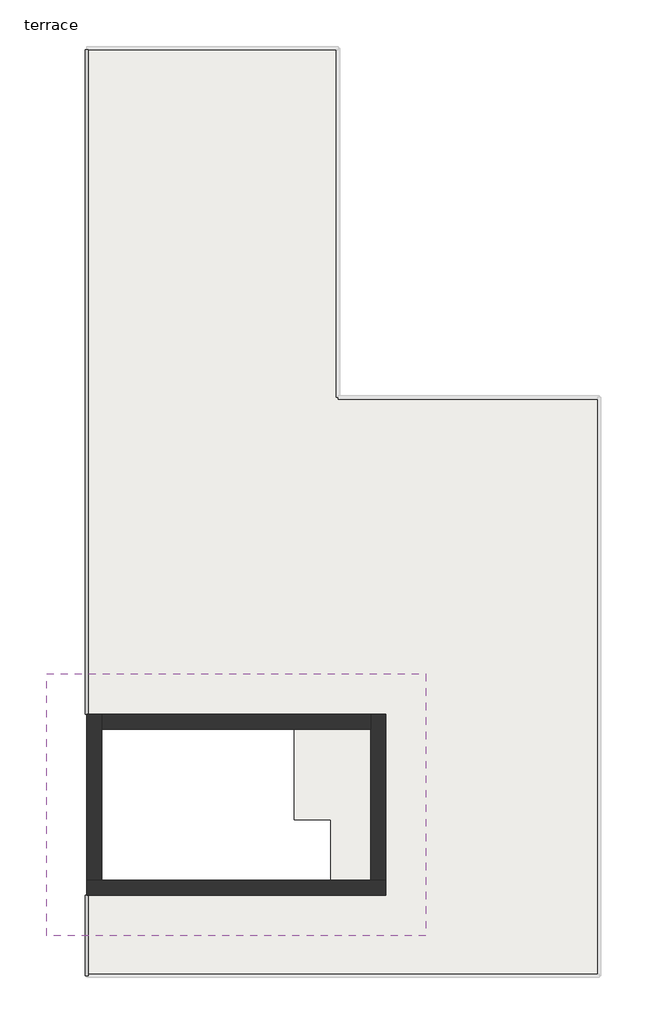
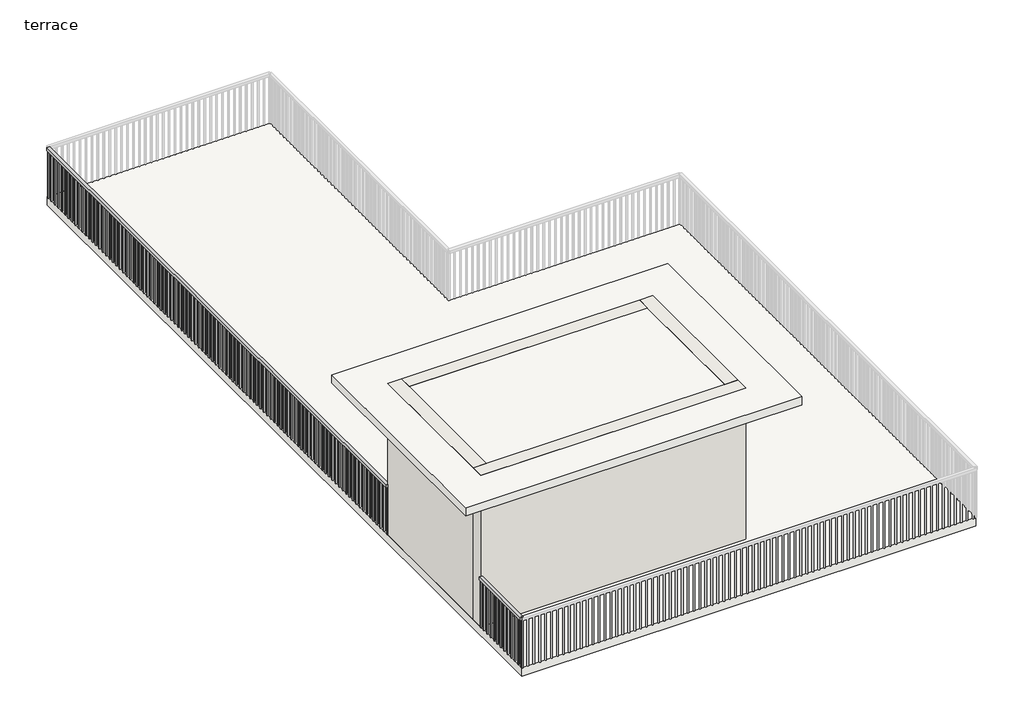
# One storey, part 1 of 4: 4 walls, 2 railings, 2 slabs.
"""IFC4 building model written with IfcOpenShell, lengths in millimetres."""

from ifc_helpers import new_model, si_unit, frame, origin, place, context, project, spatial, polyline, outline, extrude, faceted_brep, element, save

model = new_model("IFC4")

# Units and contexts
model_context = context("Model", 3, world=origin())
ifc_project = project(units=[si_unit("LENGTHUNIT", "METRE", prefix="MILLI")], contexts=[model_context])

# Site, building, storey
site = spatial("IfcSite", under=ifc_project)
building = spatial("IfcBuilding", under=site)
storey = spatial("IfcBuildingStorey", under=building, Name="terrace", Elevation=7010.4)

# Railings
placement = place(None, origin())
element("IfcRailing", 1, ObjectType="Handrail - Rectangular", at=placement, inside=storey, context=model_context, shape_type="SweptSolid", body=[
    extrude(outline(polyline([(28356.9316163, 19632.8980552), (28407.7316163, 19632.8980552), (28407.7316163, 9561.7980552), (28356.9316163, 9561.7980552), (28356.9316163, 19632.8980552)])), frame((0.0, 0.0, 7874.0), z_axis=(0.0, 0.0, 1.0), x_axis=(1.0, 0.0, 0.0)), (0.0, 0.0, 1.0), 50.8),
    extrude(outline(polyline([(28372.8066163, 9584.0230552), (28391.8566163, 9584.0230552), (28391.8566163, 9564.9730552), (28372.8066163, 9564.9730552), (28372.8066163, 9584.0230552)])), frame((0.0, 0.0, 7010.4), z_axis=(0.0, 0.0, 1.0), x_axis=(1.0, 0.0, 0.0)), (0.0, 0.0, 1.0), 863.6),
    extrude(outline(polyline([(28372.8066163, 9685.6230552), (28391.8566163, 9685.6230552), (28391.8566163, 9666.5730552), (28372.8066163, 9666.5730552), (28372.8066163, 9685.6230552)])), frame((0.0, 0.0, 7010.4), z_axis=(0.0, 0.0, 1.0), x_axis=(1.0, 0.0, 0.0)), (0.0, 0.0, 1.0), 863.6),
    extrude(outline(polyline([(28372.8066163, 9787.2230552), (28391.8566163, 9787.2230552), (28391.8566163, 9768.1730552), (28372.8066163, 9768.1730552), (28372.8066163, 9787.2230552)])), frame((0.0, 0.0, 7010.4), z_axis=(0.0, 0.0, 1.0), x_axis=(1.0, 0.0, 0.0)), (0.0, 0.0, 1.0), 863.6),
    extrude(outline(polyline([(28372.8066163, 9888.8230552), (28391.8566163, 9888.8230552), (28391.8566163, 9869.7730552), (28372.8066163, 9869.7730552), (28372.8066163, 9888.8230552)])), frame((0.0, 0.0, 7010.4), z_axis=(0.0, 0.0, 1.0), x_axis=(1.0, 0.0, 0.0)), (0.0, 0.0, 1.0), 863.6),
    extrude(outline(polyline([(28372.8066163, 9990.4230552), (28391.8566163, 9990.4230552), (28391.8566163, 9971.3730552), (28372.8066163, 9971.3730552), (28372.8066163, 9990.4230552)])), frame((0.0, 0.0, 7010.4), z_axis=(0.0, 0.0, 1.0), x_axis=(1.0, 0.0, 0.0)), (0.0, 0.0, 1.0), 863.6),
    extrude(outline(polyline([(28372.8066163, 10092.0230552), (28391.8566163, 10092.0230552), (28391.8566163, 10072.9730552), (28372.8066163, 10072.9730552), (28372.8066163, 10092.0230552)])), frame((0.0, 0.0, 7010.4), z_axis=(0.0, 0.0, 1.0), x_axis=(1.0, 0.0, 0.0)), (0.0, 0.0, 1.0), 863.6),
    extrude(outline(polyline([(28372.8066163, 10193.6230552), (28391.8566163, 10193.6230552), (28391.8566163, 10174.5730552), (28372.8066163, 10174.5730552), (28372.8066163, 10193.6230552)])), frame((0.0, 0.0, 7010.4), z_axis=(0.0, 0.0, 1.0), x_axis=(1.0, 0.0, 0.0)), (0.0, 0.0, 1.0), 863.6),
    extrude(outline(polyline([(28372.8066163, 10295.2230552), (28391.8566163, 10295.2230552), (28391.8566163, 10276.1730552), (28372.8066163, 10276.1730552), (28372.8066163, 10295.2230552)])), frame((0.0, 0.0, 7010.4), z_axis=(0.0, 0.0, 1.0), x_axis=(1.0, 0.0, 0.0)), (0.0, 0.0, 1.0), 863.6),
    extrude(outline(polyline([(28372.8066163, 10396.8230552), (28391.8566163, 10396.8230552), (28391.8566163, 10377.7730552), (28372.8066163, 10377.7730552), (28372.8066163, 10396.8230552)])), frame((0.0, 0.0, 7010.4), z_axis=(0.0, 0.0, 1.0), x_axis=(1.0, 0.0, 0.0)), (0.0, 0.0, 1.0), 863.6),
    extrude(outline(polyline([(28372.8066163, 10498.4230552), (28391.8566163, 10498.4230552), (28391.8566163, 10479.3730552), (28372.8066163, 10479.3730552), (28372.8066163, 10498.4230552)])), frame((0.0, 0.0, 7010.4), z_axis=(0.0, 0.0, 1.0), x_axis=(1.0, 0.0, 0.0)), (0.0, 0.0, 1.0), 863.6),
    extrude(outline(polyline([(28372.8066163, 10600.0230552), (28391.8566163, 10600.0230552), (28391.8566163, 10580.9730552), (28372.8066163, 10580.9730552), (28372.8066163, 10600.0230552)])), frame((0.0, 0.0, 7010.4), z_axis=(0.0, 0.0, 1.0), x_axis=(1.0, 0.0, 0.0)), (0.0, 0.0, 1.0), 863.6),
    extrude(outline(polyline([(28372.8066163, 10701.6230552), (28391.8566163, 10701.6230552), (28391.8566163, 10682.5730552), (28372.8066163, 10682.5730552), (28372.8066163, 10701.6230552)])), frame((0.0, 0.0, 7010.4), z_axis=(0.0, 0.0, 1.0), x_axis=(1.0, 0.0, 0.0)), (0.0, 0.0, 1.0), 863.6),
    extrude(outline(polyline([(28372.8066163, 10803.2230552), (28391.8566163, 10803.2230552), (28391.8566163, 10784.1730552), (28372.8066163, 10784.1730552), (28372.8066163, 10803.2230552)])), frame((0.0, 0.0, 7010.4), z_axis=(0.0, 0.0, 1.0), x_axis=(1.0, 0.0, 0.0)), (0.0, 0.0, 1.0), 863.6),
    extrude(outline(polyline([(28372.8066163, 10904.8230552), (28391.8566163, 10904.8230552), (28391.8566163, 10885.7730552), (28372.8066163, 10885.7730552), (28372.8066163, 10904.8230552)])), frame((0.0, 0.0, 7010.4), z_axis=(0.0, 0.0, 1.0), x_axis=(1.0, 0.0, 0.0)), (0.0, 0.0, 1.0), 863.6),
    extrude(outline(polyline([(28372.8066163, 11006.4230552), (28391.8566163, 11006.4230552), (28391.8566163, 10987.3730552), (28372.8066163, 10987.3730552), (28372.8066163, 11006.4230552)])), frame((0.0, 0.0, 7010.4), z_axis=(0.0, 0.0, 1.0), x_axis=(1.0, 0.0, 0.0)), (0.0, 0.0, 1.0), 863.6),
    extrude(outline(polyline([(28372.8066163, 11108.0230552), (28391.8566163, 11108.0230552), (28391.8566163, 11088.9730552), (28372.8066163, 11088.9730552), (28372.8066163, 11108.0230552)])), frame((0.0, 0.0, 7010.4), z_axis=(0.0, 0.0, 1.0), x_axis=(1.0, 0.0, 0.0)), (0.0, 0.0, 1.0), 863.6),
    extrude(outline(polyline([(28372.8066163, 11209.6230552), (28391.8566163, 11209.6230552), (28391.8566163, 11190.5730552), (28372.8066163, 11190.5730552), (28372.8066163, 11209.6230552)])), frame((0.0, 0.0, 7010.4), z_axis=(0.0, 0.0, 1.0), x_axis=(1.0, 0.0, 0.0)), (0.0, 0.0, 1.0), 863.6),
    extrude(outline(polyline([(28372.8066163, 11311.2230552), (28391.8566163, 11311.2230552), (28391.8566163, 11292.1730552), (28372.8066163, 11292.1730552), (28372.8066163, 11311.2230552)])), frame((0.0, 0.0, 7010.4), z_axis=(0.0, 0.0, 1.0), x_axis=(1.0, 0.0, 0.0)), (0.0, 0.0, 1.0), 863.6),
    extrude(outline(polyline([(28372.8066163, 11412.8230552), (28391.8566163, 11412.8230552), (28391.8566163, 11393.7730552), (28372.8066163, 11393.7730552), (28372.8066163, 11412.8230552)])), frame((0.0, 0.0, 7010.4), z_axis=(0.0, 0.0, 1.0), x_axis=(1.0, 0.0, 0.0)), (0.0, 0.0, 1.0), 863.6),
    extrude(outline(polyline([(28372.8066163, 11514.4230552), (28391.8566163, 11514.4230552), (28391.8566163, 11495.3730552), (28372.8066163, 11495.3730552), (28372.8066163, 11514.4230552)])), frame((0.0, 0.0, 7010.4), z_axis=(0.0, 0.0, 1.0), x_axis=(1.0, 0.0, 0.0)), (0.0, 0.0, 1.0), 863.6),
    extrude(outline(polyline([(28372.8066163, 11616.0230552), (28391.8566163, 11616.0230552), (28391.8566163, 11596.9730552), (28372.8066163, 11596.9730552), (28372.8066163, 11616.0230552)])), frame((0.0, 0.0, 7010.4), z_axis=(0.0, 0.0, 1.0), x_axis=(1.0, 0.0, 0.0)), (0.0, 0.0, 1.0), 863.6),
    extrude(outline(polyline([(28372.8066163, 11717.6230552), (28391.8566163, 11717.6230552), (28391.8566163, 11698.5730552), (28372.8066163, 11698.5730552), (28372.8066163, 11717.6230552)])), frame((0.0, 0.0, 7010.4), z_axis=(0.0, 0.0, 1.0), x_axis=(1.0, 0.0, 0.0)), (0.0, 0.0, 1.0), 863.6),
    extrude(outline(polyline([(28372.8066163, 11819.2230552), (28391.8566163, 11819.2230552), (28391.8566163, 11800.1730552), (28372.8066163, 11800.1730552), (28372.8066163, 11819.2230552)])), frame((0.0, 0.0, 7010.4), z_axis=(0.0, 0.0, 1.0), x_axis=(1.0, 0.0, 0.0)), (0.0, 0.0, 1.0), 863.6),
    extrude(outline(polyline([(28372.8066163, 11920.8230552), (28391.8566163, 11920.8230552), (28391.8566163, 11901.7730552), (28372.8066163, 11901.7730552), (28372.8066163, 11920.8230552)])), frame((0.0, 0.0, 7010.4), z_axis=(0.0, 0.0, 1.0), x_axis=(1.0, 0.0, 0.0)), (0.0, 0.0, 1.0), 863.6),
    extrude(outline(polyline([(28372.8066163, 12022.4230552), (28391.8566163, 12022.4230552), (28391.8566163, 12003.3730552), (28372.8066163, 12003.3730552), (28372.8066163, 12022.4230552)])), frame((0.0, 0.0, 7010.4), z_axis=(0.0, 0.0, 1.0), x_axis=(1.0, 0.0, 0.0)), (0.0, 0.0, 1.0), 863.6),
    extrude(outline(polyline([(28372.8066163, 12124.0230552), (28391.8566163, 12124.0230552), (28391.8566163, 12104.9730552), (28372.8066163, 12104.9730552), (28372.8066163, 12124.0230552)])), frame((0.0, 0.0, 7010.4), z_axis=(0.0, 0.0, 1.0), x_axis=(1.0, 0.0, 0.0)), (0.0, 0.0, 1.0), 863.6),
    extrude(outline(polyline([(28372.8066163, 12225.6230552), (28391.8566163, 12225.6230552), (28391.8566163, 12206.5730552), (28372.8066163, 12206.5730552), (28372.8066163, 12225.6230552)])), frame((0.0, 0.0, 7010.4), z_axis=(0.0, 0.0, 1.0), x_axis=(1.0, 0.0, 0.0)), (0.0, 0.0, 1.0), 863.6),
    extrude(outline(polyline([(28372.8066163, 12327.2230552), (28391.8566163, 12327.2230552), (28391.8566163, 12308.1730552), (28372.8066163, 12308.1730552), (28372.8066163, 12327.2230552)])), frame((0.0, 0.0, 7010.4), z_axis=(0.0, 0.0, 1.0), x_axis=(1.0, 0.0, 0.0)), (0.0, 0.0, 1.0), 863.6),
    extrude(outline(polyline([(28372.8066163, 12428.8230552), (28391.8566163, 12428.8230552), (28391.8566163, 12409.7730552), (28372.8066163, 12409.7730552), (28372.8066163, 12428.8230552)])), frame((0.0, 0.0, 7010.4), z_axis=(0.0, 0.0, 1.0), x_axis=(1.0, 0.0, 0.0)), (0.0, 0.0, 1.0), 863.6),
    extrude(outline(polyline([(28372.8066163, 12530.4230552), (28391.8566163, 12530.4230552), (28391.8566163, 12511.3730552), (28372.8066163, 12511.3730552), (28372.8066163, 12530.4230552)])), frame((0.0, 0.0, 7010.4), z_axis=(0.0, 0.0, 1.0), x_axis=(1.0, 0.0, 0.0)), (0.0, 0.0, 1.0), 863.6),
    extrude(outline(polyline([(28372.8066163, 12632.0230552), (28391.8566163, 12632.0230552), (28391.8566163, 12612.9730552), (28372.8066163, 12612.9730552), (28372.8066163, 12632.0230552)])), frame((0.0, 0.0, 7010.4), z_axis=(0.0, 0.0, 1.0), x_axis=(1.0, 0.0, 0.0)), (0.0, 0.0, 1.0), 863.6),
    extrude(outline(polyline([(28372.8066163, 12733.6230552), (28391.8566163, 12733.6230552), (28391.8566163, 12714.5730552), (28372.8066163, 12714.5730552), (28372.8066163, 12733.6230552)])), frame((0.0, 0.0, 7010.4), z_axis=(0.0, 0.0, 1.0), x_axis=(1.0, 0.0, 0.0)), (0.0, 0.0, 1.0), 863.6),
    extrude(outline(polyline([(28372.8066163, 12835.2230552), (28391.8566163, 12835.2230552), (28391.8566163, 12816.1730552), (28372.8066163, 12816.1730552), (28372.8066163, 12835.2230552)])), frame((0.0, 0.0, 7010.4), z_axis=(0.0, 0.0, 1.0), x_axis=(1.0, 0.0, 0.0)), (0.0, 0.0, 1.0), 863.6),
    extrude(outline(polyline([(28372.8066163, 12936.8230552), (28391.8566163, 12936.8230552), (28391.8566163, 12917.7730552), (28372.8066163, 12917.7730552), (28372.8066163, 12936.8230552)])), frame((0.0, 0.0, 7010.4), z_axis=(0.0, 0.0, 1.0), x_axis=(1.0, 0.0, 0.0)), (0.0, 0.0, 1.0), 863.6),
    extrude(outline(polyline([(28372.8066163, 13038.4230552), (28391.8566163, 13038.4230552), (28391.8566163, 13019.3730552), (28372.8066163, 13019.3730552), (28372.8066163, 13038.4230552)])), frame((0.0, 0.0, 7010.4), z_axis=(0.0, 0.0, 1.0), x_axis=(1.0, 0.0, 0.0)), (0.0, 0.0, 1.0), 863.6),
    extrude(outline(polyline([(28372.8066163, 13140.0230552), (28391.8566163, 13140.0230552), (28391.8566163, 13120.9730552), (28372.8066163, 13120.9730552), (28372.8066163, 13140.0230552)])), frame((0.0, 0.0, 7010.4), z_axis=(0.0, 0.0, 1.0), x_axis=(1.0, 0.0, 0.0)), (0.0, 0.0, 1.0), 863.6),
    extrude(outline(polyline([(28372.8066163, 13241.6230552), (28391.8566163, 13241.6230552), (28391.8566163, 13222.5730552), (28372.8066163, 13222.5730552), (28372.8066163, 13241.6230552)])), frame((0.0, 0.0, 7010.4), z_axis=(0.0, 0.0, 1.0), x_axis=(1.0, 0.0, 0.0)), (0.0, 0.0, 1.0), 863.6),
    extrude(outline(polyline([(28372.8066163, 13343.2230552), (28391.8566163, 13343.2230552), (28391.8566163, 13324.1730552), (28372.8066163, 13324.1730552), (28372.8066163, 13343.2230552)])), frame((0.0, 0.0, 7010.4), z_axis=(0.0, 0.0, 1.0), x_axis=(1.0, 0.0, 0.0)), (0.0, 0.0, 1.0), 863.6),
    extrude(outline(polyline([(28372.8066163, 13444.8230552), (28391.8566163, 13444.8230552), (28391.8566163, 13425.7730552), (28372.8066163, 13425.7730552), (28372.8066163, 13444.8230552)])), frame((0.0, 0.0, 7010.4), z_axis=(0.0, 0.0, 1.0), x_axis=(1.0, 0.0, 0.0)), (0.0, 0.0, 1.0), 863.6),
    extrude(outline(polyline([(28372.8066163, 13546.4230552), (28391.8566163, 13546.4230552), (28391.8566163, 13527.3730552), (28372.8066163, 13527.3730552), (28372.8066163, 13546.4230552)])), frame((0.0, 0.0, 7010.4), z_axis=(0.0, 0.0, 1.0), x_axis=(1.0, 0.0, 0.0)), (0.0, 0.0, 1.0), 863.6),
    extrude(outline(polyline([(28372.8066163, 13648.0230552), (28391.8566163, 13648.0230552), (28391.8566163, 13628.9730552), (28372.8066163, 13628.9730552), (28372.8066163, 13648.0230552)])), frame((0.0, 0.0, 7010.4), z_axis=(0.0, 0.0, 1.0), x_axis=(1.0, 0.0, 0.0)), (0.0, 0.0, 1.0), 863.6),
    extrude(outline(polyline([(28372.8066163, 13749.6230552), (28391.8566163, 13749.6230552), (28391.8566163, 13730.5730552), (28372.8066163, 13730.5730552), (28372.8066163, 13749.6230552)])), frame((0.0, 0.0, 7010.4), z_axis=(0.0, 0.0, 1.0), x_axis=(1.0, 0.0, 0.0)), (0.0, 0.0, 1.0), 863.6),
    extrude(outline(polyline([(28372.8066163, 13851.2230552), (28391.8566163, 13851.2230552), (28391.8566163, 13832.1730552), (28372.8066163, 13832.1730552), (28372.8066163, 13851.2230552)])), frame((0.0, 0.0, 7010.4), z_axis=(0.0, 0.0, 1.0), x_axis=(1.0, 0.0, 0.0)), (0.0, 0.0, 1.0), 863.6),
    extrude(outline(polyline([(28372.8066163, 13952.8230552), (28391.8566163, 13952.8230552), (28391.8566163, 13933.7730552), (28372.8066163, 13933.7730552), (28372.8066163, 13952.8230552)])), frame((0.0, 0.0, 7010.4), z_axis=(0.0, 0.0, 1.0), x_axis=(1.0, 0.0, 0.0)), (0.0, 0.0, 1.0), 863.6),
    extrude(outline(polyline([(28372.8066163, 14054.4230552), (28391.8566163, 14054.4230552), (28391.8566163, 14035.3730552), (28372.8066163, 14035.3730552), (28372.8066163, 14054.4230552)])), frame((0.0, 0.0, 7010.4), z_axis=(0.0, 0.0, 1.0), x_axis=(1.0, 0.0, 0.0)), (0.0, 0.0, 1.0), 863.6),
    extrude(outline(polyline([(28372.8066163, 14156.0230552), (28391.8566163, 14156.0230552), (28391.8566163, 14136.9730552), (28372.8066163, 14136.9730552), (28372.8066163, 14156.0230552)])), frame((0.0, 0.0, 7010.4), z_axis=(0.0, 0.0, 1.0), x_axis=(1.0, 0.0, 0.0)), (0.0, 0.0, 1.0), 863.6),
    extrude(outline(polyline([(28372.8066163, 14257.6230552), (28391.8566163, 14257.6230552), (28391.8566163, 14238.5730552), (28372.8066163, 14238.5730552), (28372.8066163, 14257.6230552)])), frame((0.0, 0.0, 7010.4), z_axis=(0.0, 0.0, 1.0), x_axis=(1.0, 0.0, 0.0)), (0.0, 0.0, 1.0), 863.6),
    extrude(outline(polyline([(28372.8066163, 14359.2230552), (28391.8566163, 14359.2230552), (28391.8566163, 14340.1730552), (28372.8066163, 14340.1730552), (28372.8066163, 14359.2230552)])), frame((0.0, 0.0, 7010.4), z_axis=(0.0, 0.0, 1.0), x_axis=(1.0, 0.0, 0.0)), (0.0, 0.0, 1.0), 863.6),
    extrude(outline(polyline([(28372.8066163, 14460.8230552), (28391.8566163, 14460.8230552), (28391.8566163, 14441.7730552), (28372.8066163, 14441.7730552), (28372.8066163, 14460.8230552)])), frame((0.0, 0.0, 7010.4), z_axis=(0.0, 0.0, 1.0), x_axis=(1.0, 0.0, 0.0)), (0.0, 0.0, 1.0), 863.6),
    extrude(outline(polyline([(28372.8066163, 14562.4230552), (28391.8566163, 14562.4230552), (28391.8566163, 14543.3730552), (28372.8066163, 14543.3730552), (28372.8066163, 14562.4230552)])), frame((0.0, 0.0, 7010.4), z_axis=(0.0, 0.0, 1.0), x_axis=(1.0, 0.0, 0.0)), (0.0, 0.0, 1.0), 863.6),
    extrude(outline(polyline([(28372.8066163, 14664.0230552), (28391.8566163, 14664.0230552), (28391.8566163, 14644.9730552), (28372.8066163, 14644.9730552), (28372.8066163, 14664.0230552)])), frame((0.0, 0.0, 7010.4), z_axis=(0.0, 0.0, 1.0), x_axis=(1.0, 0.0, 0.0)), (0.0, 0.0, 1.0), 863.6),
    extrude(outline(polyline([(28372.8066163, 14765.6230552), (28391.8566163, 14765.6230552), (28391.8566163, 14746.5730552), (28372.8066163, 14746.5730552), (28372.8066163, 14765.6230552)])), frame((0.0, 0.0, 7010.4), z_axis=(0.0, 0.0, 1.0), x_axis=(1.0, 0.0, 0.0)), (0.0, 0.0, 1.0), 863.6),
    extrude(outline(polyline([(28372.8066163, 14867.2230552), (28391.8566163, 14867.2230552), (28391.8566163, 14848.1730552), (28372.8066163, 14848.1730552), (28372.8066163, 14867.2230552)])), frame((0.0, 0.0, 7010.4), z_axis=(0.0, 0.0, 1.0), x_axis=(1.0, 0.0, 0.0)), (0.0, 0.0, 1.0), 863.6),
    extrude(outline(polyline([(28372.8066163, 14968.8230552), (28391.8566163, 14968.8230552), (28391.8566163, 14949.7730552), (28372.8066163, 14949.7730552), (28372.8066163, 14968.8230552)])), frame((0.0, 0.0, 7010.4), z_axis=(0.0, 0.0, 1.0), x_axis=(1.0, 0.0, 0.0)), (0.0, 0.0, 1.0), 863.6),
    extrude(outline(polyline([(28372.8066163, 15070.4230552), (28391.8566163, 15070.4230552), (28391.8566163, 15051.3730552), (28372.8066163, 15051.3730552), (28372.8066163, 15070.4230552)])), frame((0.0, 0.0, 7010.4), z_axis=(0.0, 0.0, 1.0), x_axis=(1.0, 0.0, 0.0)), (0.0, 0.0, 1.0), 863.6),
    extrude(outline(polyline([(28372.8066163, 15172.0230552), (28391.8566163, 15172.0230552), (28391.8566163, 15152.9730552), (28372.8066163, 15152.9730552), (28372.8066163, 15172.0230552)])), frame((0.0, 0.0, 7010.4), z_axis=(0.0, 0.0, 1.0), x_axis=(1.0, 0.0, 0.0)), (0.0, 0.0, 1.0), 863.6),
    extrude(outline(polyline([(28372.8066163, 15273.6230552), (28391.8566163, 15273.6230552), (28391.8566163, 15254.5730552), (28372.8066163, 15254.5730552), (28372.8066163, 15273.6230552)])), frame((0.0, 0.0, 7010.4), z_axis=(0.0, 0.0, 1.0), x_axis=(1.0, 0.0, 0.0)), (0.0, 0.0, 1.0), 863.6),
    extrude(outline(polyline([(28372.8066163, 15375.2230552), (28391.8566163, 15375.2230552), (28391.8566163, 15356.1730552), (28372.8066163, 15356.1730552), (28372.8066163, 15375.2230552)])), frame((0.0, 0.0, 7010.4), z_axis=(0.0, 0.0, 1.0), x_axis=(1.0, 0.0, 0.0)), (0.0, 0.0, 1.0), 863.6),
    extrude(outline(polyline([(28372.8066163, 15476.8230552), (28391.8566163, 15476.8230552), (28391.8566163, 15457.7730552), (28372.8066163, 15457.7730552), (28372.8066163, 15476.8230552)])), frame((0.0, 0.0, 7010.4), z_axis=(0.0, 0.0, 1.0), x_axis=(1.0, 0.0, 0.0)), (0.0, 0.0, 1.0), 863.6),
    extrude(outline(polyline([(28372.8066163, 15578.4230552), (28391.8566163, 15578.4230552), (28391.8566163, 15559.3730552), (28372.8066163, 15559.3730552), (28372.8066163, 15578.4230552)])), frame((0.0, 0.0, 7010.4), z_axis=(0.0, 0.0, 1.0), x_axis=(1.0, 0.0, 0.0)), (0.0, 0.0, 1.0), 863.6),
    extrude(outline(polyline([(28372.8066163, 15680.0230552), (28391.8566163, 15680.0230552), (28391.8566163, 15660.9730552), (28372.8066163, 15660.9730552), (28372.8066163, 15680.0230552)])), frame((0.0, 0.0, 7010.4), z_axis=(0.0, 0.0, 1.0), x_axis=(1.0, 0.0, 0.0)), (0.0, 0.0, 1.0), 863.6),
    extrude(outline(polyline([(28372.8066163, 15781.6230552), (28391.8566163, 15781.6230552), (28391.8566163, 15762.5730552), (28372.8066163, 15762.5730552), (28372.8066163, 15781.6230552)])), frame((0.0, 0.0, 7010.4), z_axis=(0.0, 0.0, 1.0), x_axis=(1.0, 0.0, 0.0)), (0.0, 0.0, 1.0), 863.6),
    extrude(outline(polyline([(28372.8066163, 15883.2230552), (28391.8566163, 15883.2230552), (28391.8566163, 15864.1730552), (28372.8066163, 15864.1730552), (28372.8066163, 15883.2230552)])), frame((0.0, 0.0, 7010.4), z_axis=(0.0, 0.0, 1.0), x_axis=(1.0, 0.0, 0.0)), (0.0, 0.0, 1.0), 863.6),
    extrude(outline(polyline([(28372.8066163, 15984.8230552), (28391.8566163, 15984.8230552), (28391.8566163, 15965.7730552), (28372.8066163, 15965.7730552), (28372.8066163, 15984.8230552)])), frame((0.0, 0.0, 7010.4), z_axis=(0.0, 0.0, 1.0), x_axis=(1.0, 0.0, 0.0)), (0.0, 0.0, 1.0), 863.6),
    extrude(outline(polyline([(28372.8066163, 16086.4230552), (28391.8566163, 16086.4230552), (28391.8566163, 16067.3730552), (28372.8066163, 16067.3730552), (28372.8066163, 16086.4230552)])), frame((0.0, 0.0, 7010.4), z_axis=(0.0, 0.0, 1.0), x_axis=(1.0, 0.0, 0.0)), (0.0, 0.0, 1.0), 863.6),
    extrude(outline(polyline([(28372.8066163, 16188.0230552), (28391.8566163, 16188.0230552), (28391.8566163, 16168.9730552), (28372.8066163, 16168.9730552), (28372.8066163, 16188.0230552)])), frame((0.0, 0.0, 7010.4), z_axis=(0.0, 0.0, 1.0), x_axis=(1.0, 0.0, 0.0)), (0.0, 0.0, 1.0), 863.6),
    extrude(outline(polyline([(28372.8066163, 16289.6230552), (28391.8566163, 16289.6230552), (28391.8566163, 16270.5730552), (28372.8066163, 16270.5730552), (28372.8066163, 16289.6230552)])), frame((0.0, 0.0, 7010.4), z_axis=(0.0, 0.0, 1.0), x_axis=(1.0, 0.0, 0.0)), (0.0, 0.0, 1.0), 863.6),
    extrude(outline(polyline([(28372.8066163, 16391.2230552), (28391.8566163, 16391.2230552), (28391.8566163, 16372.1730552), (28372.8066163, 16372.1730552), (28372.8066163, 16391.2230552)])), frame((0.0, 0.0, 7010.4), z_axis=(0.0, 0.0, 1.0), x_axis=(1.0, 0.0, 0.0)), (0.0, 0.0, 1.0), 863.6),
    extrude(outline(polyline([(28372.8066163, 16492.8230552), (28391.8566163, 16492.8230552), (28391.8566163, 16473.7730552), (28372.8066163, 16473.7730552), (28372.8066163, 16492.8230552)])), frame((0.0, 0.0, 7010.4), z_axis=(0.0, 0.0, 1.0), x_axis=(1.0, 0.0, 0.0)), (0.0, 0.0, 1.0), 863.6),
    extrude(outline(polyline([(28372.8066163, 16594.4230552), (28391.8566163, 16594.4230552), (28391.8566163, 16575.3730552), (28372.8066163, 16575.3730552), (28372.8066163, 16594.4230552)])), frame((0.0, 0.0, 7010.4), z_axis=(0.0, 0.0, 1.0), x_axis=(1.0, 0.0, 0.0)), (0.0, 0.0, 1.0), 863.6),
    extrude(outline(polyline([(28372.8066163, 16696.0230552), (28391.8566163, 16696.0230552), (28391.8566163, 16676.9730552), (28372.8066163, 16676.9730552), (28372.8066163, 16696.0230552)])), frame((0.0, 0.0, 7010.4), z_axis=(0.0, 0.0, 1.0), x_axis=(1.0, 0.0, 0.0)), (0.0, 0.0, 1.0), 863.6),
    extrude(outline(polyline([(28372.8066163, 16797.6230552), (28391.8566163, 16797.6230552), (28391.8566163, 16778.5730552), (28372.8066163, 16778.5730552), (28372.8066163, 16797.6230552)])), frame((0.0, 0.0, 7010.4), z_axis=(0.0, 0.0, 1.0), x_axis=(1.0, 0.0, 0.0)), (0.0, 0.0, 1.0), 863.6),
    extrude(outline(polyline([(28372.8066163, 16899.2230552), (28391.8566163, 16899.2230552), (28391.8566163, 16880.1730552), (28372.8066163, 16880.1730552), (28372.8066163, 16899.2230552)])), frame((0.0, 0.0, 7010.4), z_axis=(0.0, 0.0, 1.0), x_axis=(1.0, 0.0, 0.0)), (0.0, 0.0, 1.0), 863.6),
    extrude(outline(polyline([(28372.8066163, 17000.8230552), (28391.8566163, 17000.8230552), (28391.8566163, 16981.7730552), (28372.8066163, 16981.7730552), (28372.8066163, 17000.8230552)])), frame((0.0, 0.0, 7010.4), z_axis=(0.0, 0.0, 1.0), x_axis=(1.0, 0.0, 0.0)), (0.0, 0.0, 1.0), 863.6),
    extrude(outline(polyline([(28372.8066163, 17102.4230552), (28391.8566163, 17102.4230552), (28391.8566163, 17083.3730552), (28372.8066163, 17083.3730552), (28372.8066163, 17102.4230552)])), frame((0.0, 0.0, 7010.4), z_axis=(0.0, 0.0, 1.0), x_axis=(1.0, 0.0, 0.0)), (0.0, 0.0, 1.0), 863.6),
    extrude(outline(polyline([(28372.8066163, 17204.0230552), (28391.8566163, 17204.0230552), (28391.8566163, 17184.9730552), (28372.8066163, 17184.9730552), (28372.8066163, 17204.0230552)])), frame((0.0, 0.0, 7010.4), z_axis=(0.0, 0.0, 1.0), x_axis=(1.0, 0.0, 0.0)), (0.0, 0.0, 1.0), 863.6),
    extrude(outline(polyline([(28372.8066163, 17305.6230552), (28391.8566163, 17305.6230552), (28391.8566163, 17286.5730552), (28372.8066163, 17286.5730552), (28372.8066163, 17305.6230552)])), frame((0.0, 0.0, 7010.4), z_axis=(0.0, 0.0, 1.0), x_axis=(1.0, 0.0, 0.0)), (0.0, 0.0, 1.0), 863.6),
    extrude(outline(polyline([(28372.8066163, 17407.2230552), (28391.8566163, 17407.2230552), (28391.8566163, 17388.1730552), (28372.8066163, 17388.1730552), (28372.8066163, 17407.2230552)])), frame((0.0, 0.0, 7010.4), z_axis=(0.0, 0.0, 1.0), x_axis=(1.0, 0.0, 0.0)), (0.0, 0.0, 1.0), 863.6),
    extrude(outline(polyline([(28372.8066163, 17508.8230552), (28391.8566163, 17508.8230552), (28391.8566163, 17489.7730552), (28372.8066163, 17489.7730552), (28372.8066163, 17508.8230552)])), frame((0.0, 0.0, 7010.4), z_axis=(0.0, 0.0, 1.0), x_axis=(1.0, 0.0, 0.0)), (0.0, 0.0, 1.0), 863.6),
    extrude(outline(polyline([(28372.8066163, 17610.4230552), (28391.8566163, 17610.4230552), (28391.8566163, 17591.3730552), (28372.8066163, 17591.3730552), (28372.8066163, 17610.4230552)])), frame((0.0, 0.0, 7010.4), z_axis=(0.0, 0.0, 1.0), x_axis=(1.0, 0.0, 0.0)), (0.0, 0.0, 1.0), 863.6),
    extrude(outline(polyline([(28372.8066163, 17712.0230552), (28391.8566163, 17712.0230552), (28391.8566163, 17692.9730552), (28372.8066163, 17692.9730552), (28372.8066163, 17712.0230552)])), frame((0.0, 0.0, 7010.4), z_axis=(0.0, 0.0, 1.0), x_axis=(1.0, 0.0, 0.0)), (0.0, 0.0, 1.0), 863.6),
    extrude(outline(polyline([(28372.8066163, 17813.6230552), (28391.8566163, 17813.6230552), (28391.8566163, 17794.5730552), (28372.8066163, 17794.5730552), (28372.8066163, 17813.6230552)])), frame((0.0, 0.0, 7010.4), z_axis=(0.0, 0.0, 1.0), x_axis=(1.0, 0.0, 0.0)), (0.0, 0.0, 1.0), 863.6),
    extrude(outline(polyline([(28372.8066163, 17915.2230552), (28391.8566163, 17915.2230552), (28391.8566163, 17896.1730552), (28372.8066163, 17896.1730552), (28372.8066163, 17915.2230552)])), frame((0.0, 0.0, 7010.4), z_axis=(0.0, 0.0, 1.0), x_axis=(1.0, 0.0, 0.0)), (0.0, 0.0, 1.0), 863.6),
    extrude(outline(polyline([(28372.8066163, 18016.8230552), (28391.8566163, 18016.8230552), (28391.8566163, 17997.7730552), (28372.8066163, 17997.7730552), (28372.8066163, 18016.8230552)])), frame((0.0, 0.0, 7010.4), z_axis=(0.0, 0.0, 1.0), x_axis=(1.0, 0.0, 0.0)), (0.0, 0.0, 1.0), 863.6),
    extrude(outline(polyline([(28372.8066163, 18118.4230552), (28391.8566163, 18118.4230552), (28391.8566163, 18099.3730552), (28372.8066163, 18099.3730552), (28372.8066163, 18118.4230552)])), frame((0.0, 0.0, 7010.4), z_axis=(0.0, 0.0, 1.0), x_axis=(1.0, 0.0, 0.0)), (0.0, 0.0, 1.0), 863.6),
    extrude(outline(polyline([(28372.8066163, 18220.0230552), (28391.8566163, 18220.0230552), (28391.8566163, 18200.9730552), (28372.8066163, 18200.9730552), (28372.8066163, 18220.0230552)])), frame((0.0, 0.0, 7010.4), z_axis=(0.0, 0.0, 1.0), x_axis=(1.0, 0.0, 0.0)), (0.0, 0.0, 1.0), 863.6),
    extrude(outline(polyline([(28372.8066163, 18321.6230552), (28391.8566163, 18321.6230552), (28391.8566163, 18302.5730552), (28372.8066163, 18302.5730552), (28372.8066163, 18321.6230552)])), frame((0.0, 0.0, 7010.4), z_axis=(0.0, 0.0, 1.0), x_axis=(1.0, 0.0, 0.0)), (0.0, 0.0, 1.0), 863.6),
    extrude(outline(polyline([(28372.8066163, 18423.2230552), (28391.8566163, 18423.2230552), (28391.8566163, 18404.1730552), (28372.8066163, 18404.1730552), (28372.8066163, 18423.2230552)])), frame((0.0, 0.0, 7010.4), z_axis=(0.0, 0.0, 1.0), x_axis=(1.0, 0.0, 0.0)), (0.0, 0.0, 1.0), 863.6),
    extrude(outline(polyline([(28372.8066163, 18524.8230552), (28391.8566163, 18524.8230552), (28391.8566163, 18505.7730552), (28372.8066163, 18505.7730552), (28372.8066163, 18524.8230552)])), frame((0.0, 0.0, 7010.4), z_axis=(0.0, 0.0, 1.0), x_axis=(1.0, 0.0, 0.0)), (0.0, 0.0, 1.0), 863.6),
    extrude(outline(polyline([(28372.8066163, 18626.4230552), (28391.8566163, 18626.4230552), (28391.8566163, 18607.3730552), (28372.8066163, 18607.3730552), (28372.8066163, 18626.4230552)])), frame((0.0, 0.0, 7010.4), z_axis=(0.0, 0.0, 1.0), x_axis=(1.0, 0.0, 0.0)), (0.0, 0.0, 1.0), 863.6),
    extrude(outline(polyline([(28372.8066163, 18728.0230552), (28391.8566163, 18728.0230552), (28391.8566163, 18708.9730552), (28372.8066163, 18708.9730552), (28372.8066163, 18728.0230552)])), frame((0.0, 0.0, 7010.4), z_axis=(0.0, 0.0, 1.0), x_axis=(1.0, 0.0, 0.0)), (0.0, 0.0, 1.0), 863.6),
    extrude(outline(polyline([(28372.8066163, 18829.6230552), (28391.8566163, 18829.6230552), (28391.8566163, 18810.5730552), (28372.8066163, 18810.5730552), (28372.8066163, 18829.6230552)])), frame((0.0, 0.0, 7010.4), z_axis=(0.0, 0.0, 1.0), x_axis=(1.0, 0.0, 0.0)), (0.0, 0.0, 1.0), 863.6),
    extrude(outline(polyline([(28372.8066163, 18931.2230552), (28391.8566163, 18931.2230552), (28391.8566163, 18912.1730552), (28372.8066163, 18912.1730552), (28372.8066163, 18931.2230552)])), frame((0.0, 0.0, 7010.4), z_axis=(0.0, 0.0, 1.0), x_axis=(1.0, 0.0, 0.0)), (0.0, 0.0, 1.0), 863.6),
    extrude(outline(polyline([(28372.8066163, 19032.8230552), (28391.8566163, 19032.8230552), (28391.8566163, 19013.7730552), (28372.8066163, 19013.7730552), (28372.8066163, 19032.8230552)])), frame((0.0, 0.0, 7010.4), z_axis=(0.0, 0.0, 1.0), x_axis=(1.0, 0.0, 0.0)), (0.0, 0.0, 1.0), 863.6),
    extrude(outline(polyline([(28372.8066163, 19134.4230552), (28391.8566163, 19134.4230552), (28391.8566163, 19115.3730552), (28372.8066163, 19115.3730552), (28372.8066163, 19134.4230552)])), frame((0.0, 0.0, 7010.4), z_axis=(0.0, 0.0, 1.0), x_axis=(1.0, 0.0, 0.0)), (0.0, 0.0, 1.0), 863.6),
    extrude(outline(polyline([(28372.8066163, 19236.0230552), (28391.8566163, 19236.0230552), (28391.8566163, 19216.9730552), (28372.8066163, 19216.9730552), (28372.8066163, 19236.0230552)])), frame((0.0, 0.0, 7010.4), z_axis=(0.0, 0.0, 1.0), x_axis=(1.0, 0.0, 0.0)), (0.0, 0.0, 1.0), 863.6),
    extrude(outline(polyline([(28372.8066163, 19337.6230552), (28391.8566163, 19337.6230552), (28391.8566163, 19318.5730552), (28372.8066163, 19318.5730552), (28372.8066163, 19337.6230552)])), frame((0.0, 0.0, 7010.4), z_axis=(0.0, 0.0, 1.0), x_axis=(1.0, 0.0, 0.0)), (0.0, 0.0, 1.0), 863.6),
    extrude(outline(polyline([(28372.8066163, 19439.2230552), (28391.8566163, 19439.2230552), (28391.8566163, 19420.1730552), (28372.8066163, 19420.1730552), (28372.8066163, 19439.2230552)])), frame((0.0, 0.0, 7010.4), z_axis=(0.0, 0.0, 1.0), x_axis=(1.0, 0.0, 0.0)), (0.0, 0.0, 1.0), 863.6),
    extrude(outline(polyline([(28372.8066163, 19540.8230552), (28391.8566163, 19540.8230552), (28391.8566163, 19521.7730552), (28372.8066163, 19521.7730552), (28372.8066163, 19540.8230552)])), frame((0.0, 0.0, 7010.4), z_axis=(0.0, 0.0, 1.0), x_axis=(1.0, 0.0, 0.0)), (0.0, 0.0, 1.0), 863.6),
    extrude(outline(polyline([(28372.8066163, 9580.8480552), (28391.8566163, 9580.8480552), (28391.8566163, 9561.7980552), (28372.8066163, 9561.7980552), (28372.8066163, 9580.8480552)])), frame((0.0, 0.0, 7010.4), z_axis=(0.0, 0.0, 1.0), x_axis=(1.0, 0.0, 0.0)), (0.0, 0.0, 1.0), 863.6),
    extrude(outline(polyline([(28372.8066163, 19632.8980552), (28391.8566163, 19632.8980552), (28391.8566163, 19613.8480552), (28372.8066163, 19613.8480552), (28372.8066163, 19632.8980552)])), frame((0.0, 0.0, 7010.4), z_axis=(0.0, 0.0, 1.0), x_axis=(1.0, 0.0, 0.0)), (0.0, 0.0, 1.0), 863.6),
])
element("IfcRailing", 2, ObjectType="Handrail - Rectangular", at=placement, inside=storey, context=model_context, shape_type="SweptSolid", body=[
    extrude(outline(polyline([(28407.7316163, 5593.0480552), (28356.9316163, 5593.0480552), (28356.9316163, 6812.2480552), (28407.7316163, 6812.2480552), (28407.7316163, 5593.0480552)])), frame((0.0, 0.0, 7874.0), z_axis=(0.0, 0.0, 1.0), x_axis=(1.0, 0.0, 0.0)), (0.0, 0.0, 1.0), 50.8),
    extrude(outline(polyline([(28391.8566163, 6701.1230552), (28372.8066163, 6701.1230552), (28372.8066163, 6720.1730552), (28391.8566163, 6720.1730552), (28391.8566163, 6701.1230552)])), frame((0.0, 0.0, 7010.4), z_axis=(0.0, 0.0, 1.0), x_axis=(1.0, 0.0, 0.0)), (0.0, 0.0, 1.0), 863.6),
    extrude(outline(polyline([(28391.8566163, 6599.5230552), (28372.8066163, 6599.5230552), (28372.8066163, 6618.5730552), (28391.8566163, 6618.5730552), (28391.8566163, 6599.5230552)])), frame((0.0, 0.0, 7010.4), z_axis=(0.0, 0.0, 1.0), x_axis=(1.0, 0.0, 0.0)), (0.0, 0.0, 1.0), 863.6),
    extrude(outline(polyline([(28391.8566163, 6497.9230552), (28372.8066163, 6497.9230552), (28372.8066163, 6516.9730552), (28391.8566163, 6516.9730552), (28391.8566163, 6497.9230552)])), frame((0.0, 0.0, 7010.4), z_axis=(0.0, 0.0, 1.0), x_axis=(1.0, 0.0, 0.0)), (0.0, 0.0, 1.0), 863.6),
    extrude(outline(polyline([(28391.8566163, 6396.3230552), (28372.8066163, 6396.3230552), (28372.8066163, 6415.3730552), (28391.8566163, 6415.3730552), (28391.8566163, 6396.3230552)])), frame((0.0, 0.0, 7010.4), z_axis=(0.0, 0.0, 1.0), x_axis=(1.0, 0.0, 0.0)), (0.0, 0.0, 1.0), 863.6),
    extrude(outline(polyline([(28391.8566163, 6294.7230552), (28372.8066163, 6294.7230552), (28372.8066163, 6313.7730552), (28391.8566163, 6313.7730552), (28391.8566163, 6294.7230552)])), frame((0.0, 0.0, 7010.4), z_axis=(0.0, 0.0, 1.0), x_axis=(1.0, 0.0, 0.0)), (0.0, 0.0, 1.0), 863.6),
    extrude(outline(polyline([(28391.8566163, 6193.1230552), (28372.8066163, 6193.1230552), (28372.8066163, 6212.1730552), (28391.8566163, 6212.1730552), (28391.8566163, 6193.1230552)])), frame((0.0, 0.0, 7010.4), z_axis=(0.0, 0.0, 1.0), x_axis=(1.0, 0.0, 0.0)), (0.0, 0.0, 1.0), 863.6),
    extrude(outline(polyline([(28391.8566163, 6091.5230552), (28372.8066163, 6091.5230552), (28372.8066163, 6110.5730552), (28391.8566163, 6110.5730552), (28391.8566163, 6091.5230552)])), frame((0.0, 0.0, 7010.4), z_axis=(0.0, 0.0, 1.0), x_axis=(1.0, 0.0, 0.0)), (0.0, 0.0, 1.0), 863.6),
    extrude(outline(polyline([(28391.8566163, 5989.9230552), (28372.8066163, 5989.9230552), (28372.8066163, 6008.9730552), (28391.8566163, 6008.9730552), (28391.8566163, 5989.9230552)])), frame((0.0, 0.0, 7010.4), z_axis=(0.0, 0.0, 1.0), x_axis=(1.0, 0.0, 0.0)), (0.0, 0.0, 1.0), 863.6),
    extrude(outline(polyline([(28391.8566163, 5888.3230552), (28372.8066163, 5888.3230552), (28372.8066163, 5907.3730552), (28391.8566163, 5907.3730552), (28391.8566163, 5888.3230552)])), frame((0.0, 0.0, 7010.4), z_axis=(0.0, 0.0, 1.0), x_axis=(1.0, 0.0, 0.0)), (0.0, 0.0, 1.0), 863.6),
    extrude(outline(polyline([(28391.8566163, 5786.7230552), (28372.8066163, 5786.7230552), (28372.8066163, 5805.7730552), (28391.8566163, 5805.7730552), (28391.8566163, 5786.7230552)])), frame((0.0, 0.0, 7010.4), z_axis=(0.0, 0.0, 1.0), x_axis=(1.0, 0.0, 0.0)), (0.0, 0.0, 1.0), 863.6),
    extrude(outline(polyline([(28391.8566163, 5685.1230552), (28372.8066163, 5685.1230552), (28372.8066163, 5704.1730552), (28391.8566163, 5704.1730552), (28391.8566163, 5685.1230552)])), frame((0.0, 0.0, 7010.4), z_axis=(0.0, 0.0, 1.0), x_axis=(1.0, 0.0, 0.0)), (0.0, 0.0, 1.0), 863.6),
    extrude(outline(polyline([(28391.8566163, 6793.1980552), (28372.8066163, 6793.1980552), (28372.8066163, 6812.2480552), (28391.8566163, 6812.2480552), (28391.8566163, 6793.1980552)])), frame((0.0, 0.0, 7010.4), z_axis=(0.0, 0.0, 1.0), x_axis=(1.0, 0.0, 0.0)), (0.0, 0.0, 1.0), 863.6),
    extrude(outline(polyline([(28391.8566163, 5593.0480552), (28372.8066163, 5593.0480552), (28372.8066163, 5612.0980552), (28391.8566163, 5612.0980552), (28391.8566163, 5593.0480552)])), frame((0.0, 0.0, 7010.4), z_axis=(0.0, 0.0, 1.0), x_axis=(1.0, 0.0, 0.0)), (0.0, 0.0, 1.0), 863.6),
])

# Slabs
element("IfcSlab", 3, ObjectType="Generic - 12\" 2", at=placement, inside=storey, context=model_context, shape_type="SweptSolid", body=[
    extrude(outline(polyline([(33526.1451197, 10171.3980552), (33526.1451197, 6202.6480552), (27772.7316163, 6202.6480552), (27772.7316163, 10171.3980552), (33526.1451197, 10171.3980552)])), frame((0.0, 0.0, 9601.2), z_axis=(0.0, 0.0, 1.0), x_axis=(1.0, 0.0, 0.0)), (0.0, 0.0, 1.0), 152.4),
])
element("IfcSlab", 4, ObjectType="Generic - 12\" 3", at=placement, inside=storey, context=model_context, shape_type="SweptSolid", body=[
    extrude(outline(polyline([(32192.3316163, 19658.2980552), (32192.3316163, 14362.3980552), (36154.7316163, 14362.3980552), (36154.7316163, 5593.0480552), (28382.3316163, 5593.0480552), (28382.3316163, 19658.2980552), (32192.3316163, 19658.2980552)]), holes=[polyline([(31519.2316163, 7955.2480552), (31519.2316163, 9333.1980552), (28610.9316163, 9333.1980552), (28610.9316163, 7040.8480552), (32078.0316163, 7040.8480552), (32078.0316163, 7955.2480552), (31519.2316163, 7955.2480552)])]), frame((0.0, 0.0, 6858.0), z_axis=(0.0, 0.0, 1.0), x_axis=(1.0, 0.0, 0.0)), (0.0, 0.0, 1.0), 152.4),
])

# Walls
element("IfcWall", 5, ObjectType="Generic - 9\"", at=placement, inside=storey, context=model_context, shape_type="Brep", body=[
    faceted_brep([(28382.3316163, 6812.2480552, 7010.4), (32916.5451197, 6812.2480552, 7010.4), (32916.5451197, 6812.2480552, 9753.6), (28382.3316163, 6812.2480552, 9753.6), (28382.3316163, 7040.8480552, 7010.4), (28382.3316163, 7040.8480552, 9753.6), (28610.9316163, 7040.8480552, 9753.6), (32687.9451197, 7040.8480552, 9753.6), (32916.5451197, 7040.8480552, 9753.6), (32916.5451197, 7040.8480552, 7010.4), (32687.9451197, 7040.8480552, 7010.4), (28610.9316163, 7040.8480552, 7010.4)], [[[0, 1, 2, 3]], [[4, 5, 6, 7, 8, 9, 10, 11]], [[1, 0, 4, 11, 10, 9]], [[3, 2, 8, 7, 6, 5]], [[2, 1, 9, 8]], [[0, 3, 5, 4]]]),
])
element("IfcWall", 6, ObjectType="Generic - 9\"", at=placement, inside=storey, context=model_context, shape_type="Brep", body=[
    faceted_brep([(32916.5451197, 7040.8480552, 7010.4), (32916.5451197, 9561.7980552, 7010.4), (32916.5451197, 9561.7980552, 9753.6), (32916.5451197, 7040.8480552, 9753.6), (32687.9451197, 7040.8480552, 7010.4), (32687.9451197, 7040.8480552, 9753.6), (32687.9451197, 9333.1980552, 9753.6), (32687.9451197, 9561.7980552, 9753.6), (32687.9451197, 9561.7980552, 7010.4), (32687.9451197, 9333.1980552, 7010.4)], [[[0, 1, 2, 3]], [[4, 5, 6, 7, 8, 9]], [[1, 0, 4, 9, 8]], [[3, 2, 7, 6, 5]], [[0, 3, 5, 4]], [[2, 1, 8, 7]]]),
])
element("IfcWall", 7, ObjectType="Generic - 9\"", at=placement, inside=storey, context=model_context, shape_type="Brep", body=[
    faceted_brep([(28610.9316163, 7040.8480552, 7010.4), (28610.9316163, 9333.1980552, 7010.4), (28610.9316163, 9561.7980552, 7010.4), (28610.9316163, 9561.7980552, 9753.6), (28610.9316163, 9333.1980552, 9753.6), (28610.9316163, 7040.8480552, 9753.6), (28382.3316163, 7040.8480552, 7010.4), (28382.3316163, 7040.8480552, 9753.6), (28382.3316163, 9561.7980552, 9753.6), (28382.3316163, 9561.7980552, 7010.4)], [[[0, 1, 2, 3, 4, 5]], [[6, 7, 8, 9]], [[2, 1, 0, 6, 9]], [[5, 4, 3, 8, 7]], [[0, 5, 7, 6]], [[3, 2, 9, 8]]]),
])
element("IfcWall", 8, ObjectType="Generic - 9\"", at=placement, inside=storey, context=model_context, shape_type="SweptSolid", body=[
    extrude(outline(polyline([(32687.9451197, 9333.1980552), (28610.9316163, 9333.1980552), (28610.9316163, 9561.7980552), (32687.9451197, 9561.7980552), (32687.9451197, 9333.1980552)])), frame((0.0, 0.0, 7010.4), z_axis=(0.0, 0.0, 1.0), x_axis=(1.0, 0.0, 0.0)), (0.0, 0.0, 1.0), 2743.2),
])

save(model, "model.ifc")

# Revit data of these elements
# Type "Handrail - Rectangular"
#   Assembly Code = "C2010400"
#   built-in parameter 1008612 = 0.0416667 (stored number, unit not read)
#   built-in parameter 1008611 = 0.0416667 (stored number, unit not read)
#   built-in parameter 1008609 = 0.333333 (stored number, unit not read)
#   built-in parameter 1008604 = 0.166667 (stored number, unit not read)
#   built-in parameter 1008603 = 0.166667 (stored number, unit not read)
#   Railing Height = 3' - 0"
#   built-in parameter 1008630 = 2
#   built-in parameter 1008610 = 2
#   built-in parameter 1008618 = Baluster - Square : 3/4"
# Type "Generic - 12\" 2"
#   Assembly Code = "B1010"
#   Function = 0
#   Layers, outside or top first: 0' - 6" no material (function 1)
# Type "Generic - 12\" 3"
#   Assembly Code = "B1010"
#   Function = 0
#   Layers, outside or top first: 0' - 6" no material (function 1)
# Type "Generic - 9\""
#   Assembly Code = "B2010"
#   Layers, outside or top first: 0' - 9" no material (function 1)
# Elements 1, 2 (IfcRailing, "Handrail - Rectangular")
#   Phase Created = New Construction
# Element 3 (IfcSlab, "Generic - 12\" 2")
#   Height Offset From Level = 9' - 0"
#   Phase Created = New Construction
#   Materials on its faces: "Default Floor"
# Element 4 (IfcSlab, "Generic - 12\" 3")
#   Height Offset From Level = 0' - 0"
#   Phase Created = New Construction
#   Materials on its faces: "Default Floor"
# Elements 5, 6, 7, 8 (IfcWall, "Generic - 9\"")
#   Top Offset = 0' - 0"
#   Base Offset = 0' - 0"
#   Unconnected Height = 9' - 0"
#   wall height = 9' - 0"
#   Phase Created = New Construction
#   Base Constraint = terrace
#   Materials on its faces: "Default Wall"
# Materials
#   "Default Floor": colour RGB 128 128 128, transparency 0, Cost = 0
#   "Default Wall": colour RGB 128 128 128, transparency 0, Cost = 0
